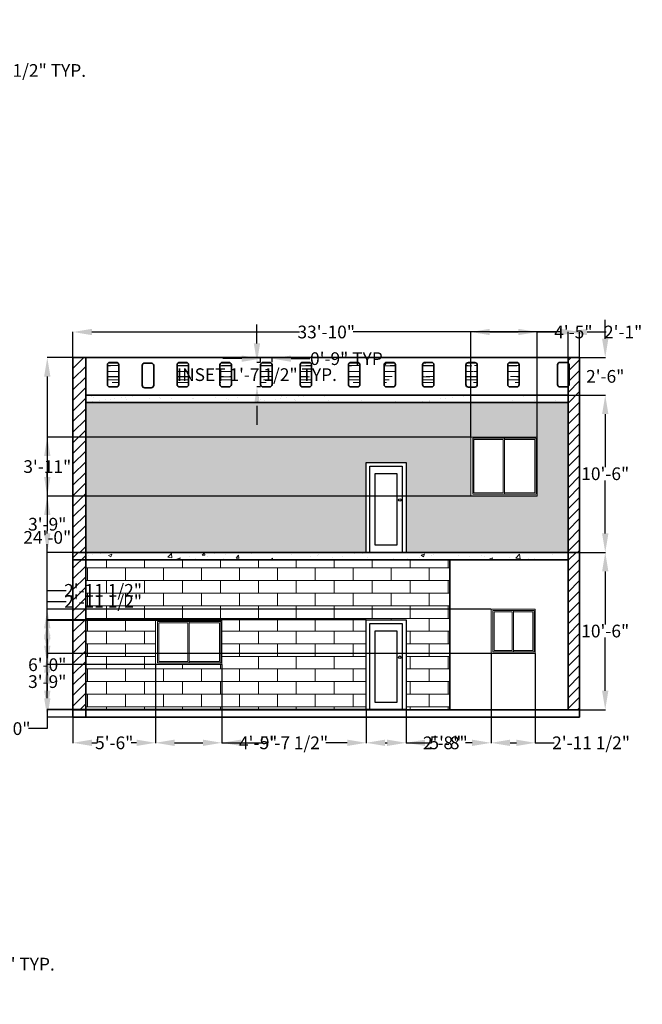
# Model space of a CAD drawing. Units: inches. Extents: x -2 to 7298, y -2 to 4583.
# Tile 6 of 6: x 6799 to 7298, y 3778 to 4567. Entities that reach past the tile are written whole.
import ezdxf

# ---------------------------------------------------------------- set-up
doc = ezdxf.new("R2010")
doc.units = ezdxf.units.IN
doc.header["$MEASUREMENT"] = 0
for name, color, linetype, lineweight in [('A-ANNO-DIMS', 2, 'Continuous', 18), ('A-ELEV', 7, 'Continuous', 35), ('A-ELEV-DOOR', 4, 'Continuous', 25), ('A-ELEV-GLAZ', 4, 'Continuous', 18), ('A-ELEV-PATT', 252, 'Continuous', 13)]:
    doc.layers.add(name, color=color, linetype=linetype, lineweight=lineweight)
doc.styles.get("Standard").update_dxf_attribs({"font": 'arial.ttf'})
doc.dimstyles.get("Standard").update_dxf_attribs({"dimtxt": 10.18, "dimasz": 15.18, "dimexe": 0.18, "dimexo": 0.0625, "dimgap": 0.09, "dimtad": 0, "dimtih": 1, "dimtoh": 1, "dimdec": 0, "dimzin": 0, "dimdsep": 46, "dimlunit": 3, "dimtxsty": 'Standard', "dimcen": 0.09, "dimadec": 0, "dimazin": 0, "dimtfac": 1, "dimtdec": 0, "dimtofl": 0, "dimtmove": 0, "dimatfit": 3, "dimfxl": 1, "dimtolj": 1, "dimtzin": 0, "dimarcsym": 0})

# ---------------------------------------------------------------- blocks, each defined once
blk = doc.blocks.new('*U14')
for p, q in [((38.1, 38.1), (38.1, 876.3)), ((38.1, 876.3), (682.2, 876.3)), ((682.2, 38.1), (682.2, 876.3)), ((682.2, 876.3), (1326.3, 876.3)), ((1326.3, 876.3), (1326.3, 38.1)), ((682.2, 38.1), (38.1, 38.1)), ((1326.3, 38.1), (682.2, 38.1))]:
    blk.add_line(p, q)
blk.add_lwpolyline([(0, 0), (1350, 0), (1350, 900), (0, 900)], close=True)
for points in [[(656.8, 850.9), (656.8, 63.5), (63.5, 63.5), (63.5, 850.9), (656.8, 850.9)], [(682.2, 850.9), (1300.9, 850.9), (1300.9, 63.5), (682.2, 63.5)]]:
    blk.add_lwpolyline(points)
blk = doc.blocks.new('*U17')
blk.add_lwpolyline([(3.12, 0.01), (0.12, 0.01), (0.12, 72.01), (32.12, 72.01), (32.12, 0.01), (29.12, 0.01)])
for points in [[(29.12, 68.99), (29.12, 0.01), (3.12, 0.01), (3.12, 68.99)], [(25.12, 6.01), (25.12, 62.99), (7.12, 62.99), (7.12, 6.01)]]:
    blk.add_lwpolyline(points, close=True)
blk.add_circle((27.12, 42.01), 1)
blk = doc.blocks.new('*U18')
for p, q in [((38.1, 38.1), (38.1, 876.3)), ((38.1, 876.3), (457.2, 876.3)), ((457.2, 38.1), (457.2, 876.3)), ((457.2, 876.3), (876.3, 876.3)), ((876.3, 876.3), (876.3, 38.1)), ((457.2, 38.1), (38.1, 38.1)), ((876.3, 38.1), (457.2, 38.1))]:
    blk.add_line(p, q)
blk.add_lwpolyline([(0, 0), (900, 0), (900, 900), (0, 900)], close=True)
for points in [[(431.8, 850.9), (431.8, 63.5), (63.5, 63.5), (63.5, 850.9), (431.8, 850.9)], [(457.2, 850.9), (850.9, 850.9), (850.9, 63.5), (457.2, 63.5)]]:
    blk.add_lwpolyline(points)
blk = doc.blocks.new('*U19')
for p, q in [((38.1, 38.1), (38.1, 1176.3)), ((38.1, 1176.3), (682.2, 1176.3)), ((682.2, 38.1), (682.2, 1176.3)), ((682.2, 1176.3), (1326.3, 1176.3)), ((1326.3, 1176.3), (1326.3, 38.1)), ((682.2, 38.1), (38.1, 38.1)), ((1326.3, 38.1), (682.2, 38.1))]:
    blk.add_line(p, q)
blk.add_lwpolyline([(0, 0), (1350, 0), (1350, 1200), (0, 1200)], close=True)
for points in [[(656.8, 1150.9), (656.8, 63.5), (63.5, 63.5), (63.5, 1150.9), (656.8, 1150.9)], [(682.2, 1150.9), (1300.9, 1150.9), (1300.9, 63.5), (682.2, 63.5)]]:
    blk.add_lwpolyline(points)
blk = doc.blocks.new('PARAPET-INSET')
blk.add_lwpolyline([(0, 17.72, -0.414214), (2, 19.72), (7.14, 19.72, -0.414214), (9.14, 17.72), (9.14, 2, -0.414214), (7.14, 0), (2, 0, -0.414214), (0, 2)], format="xyb", close=True)
blk = doc.blocks.new('*D33')
at = {"layer": 'A-ANNO-DIMS', "color": 0, "lineweight": -2, "transparency": 16777216}
for p, q in [((6989.04, 4307.74), (6989.04, 4322.92)), ((6991.93, 4292.56), (6988.86, 4292.56)), ((6991.93, 4272.84), (6988.86, 4272.84)), ((6989.04, 4257.66), (6989.04, 4242.48))]:
    blk.add_line(p, q, dxfattribs=at)
at = {"layer": 'A-ANNO-DIMS', "color": 0, "transparency": 16777216}
for points in [[(6986.51, 4307.74), (6991.57, 4307.74), (6989.04, 4292.56)], [(6986.51, 4257.66), (6991.57, 4257.66), (6989.04, 4272.84)]]:
    blk.add_solid(points, dxfattribs=at)
at = {"layer": 'Defpoints', "color": 0, "transparency": 16777216}
for p in [(6989.04, 4292.56), (6991.99, 4292.56), (6991.99, 4272.84)]:
    blk.add_point(p, dxfattribs=at)
at = {"layer": 'A-ANNO-DIMS', "color": 0, "transparency": 16777216, "insert": (6989.04, 4282.7), "char_height": 10.18, "attachment_point": 5}
blk.add_mtext('\\A1;INSET 1\'-7 1/2" TYP.', dxfattribs=at)
blk = doc.blocks.new('*D34')
at = {"layer": 'A-ANNO-DIMS', "color": 0, "lineweight": -2, "transparency": 16777216}
for p, q in [((6976.81, 4295.52), (6961.63, 4295.52)), ((6991.99, 4292.62), (6991.99, 4295.7)), ((7001.14, 4292.62), (7001.14, 4295.7)), ((7016.32, 4295.52), (7031.5, 4295.52))]:
    blk.add_line(p, q, dxfattribs=at)
at = {"layer": 'A-ANNO-DIMS', "color": 0, "transparency": 16777216}
for points in [[(6976.81, 4298.05), (6976.81, 4292.99), (6991.99, 4295.52)], [(7016.32, 4298.05), (7016.32, 4292.99), (7001.14, 4295.52)]]:
    blk.add_solid(points, dxfattribs=at)
at = {"layer": 'Defpoints', "color": 0, "transparency": 16777216}
for p in [(6991.99, 4292.56), (7001.14, 4295.52), (7001.14, 4292.56)]:
    blk.add_point(p, dxfattribs=at)
at = {"layer": 'A-ANNO-DIMS', "color": 0, "transparency": 16777216, "insert": (7062.62, 4295.52), "char_height": 10.18, "attachment_point": 5}
blk.add_mtext('\\A1;0\'-9" TYP.', dxfattribs=at)
blk = doc.blocks.new('*D45')
at = {"layer": 'A-ANNO-DIMS', "color": 0, "lineweight": -2, "transparency": 16777216}
for p, q in [((6628.99, 3810.47), (6613.81, 3810.47)), ((6644.17, 3809.69), (6644.17, 3810.65)), ((6649.81, 3809.69), (6649.81, 3810.65)), ((6664.99, 3810.47), (6680.17, 3810.47))]:
    blk.add_line(p, q, dxfattribs=at)
at = {"layer": 'A-ANNO-DIMS', "color": 0, "transparency": 16777216}
for points in [[(6628.99, 3813), (6628.99, 3807.94), (6644.17, 3810.47)], [(6664.99, 3813), (6664.99, 3807.94), (6649.81, 3810.47)]]:
    blk.add_solid(points, dxfattribs=at)
at = {"layer": 'Defpoints', "color": 0, "transparency": 16777216}
for p in [(6649.81, 3810.47), (6644.17, 3809.63), (6649.81, 3809.63)]:
    blk.add_point(p, dxfattribs=at)
at = {"layer": 'A-ANNO-DIMS', "color": 0, "transparency": 16777216, "insert": (6754.93, 3810.47), "char_height": 10.18, "attachment_point": 5}
blk.add_mtext('\\A1;BURNER 0\'-5 1/2" TYP.', dxfattribs=at)
blk = doc.blocks.new('*D53')
at = {"layer": 'A-ANNO-DIMS', "color": 0, "lineweight": -2, "transparency": 16777216}
for p, q in [((6616.96, 4528.32), (6616.96, 4526.19)), ((6630.33, 4528.32), (6630.33, 4526.19)), ((6601.78, 4526.37), (6586.6, 4526.37)), ((6645.51, 4526.37), (6660.69, 4526.37))]:
    blk.add_line(p, q, dxfattribs=at)
at = {"layer": 'A-ANNO-DIMS', "color": 0, "transparency": 16777216}
for points in [[(6601.78, 4528.9), (6601.78, 4523.84), (6616.96, 4526.37)], [(6645.51, 4528.9), (6645.51, 4523.84), (6630.33, 4526.37)]]:
    blk.add_solid(points, dxfattribs=at)
at = {"layer": 'Defpoints', "color": 0, "transparency": 16777216}
for p in [(6616.96, 4528.38), (6630.33, 4528.38), (6630.33, 4526.37)]:
    blk.add_point(p, dxfattribs=at)
at = {"layer": 'A-ANNO-DIMS', "color": 0, "transparency": 16777216, "insert": (6758.34, 4526.37), "char_height": 10.18, "attachment_point": 5}
blk.add_mtext('\\A1;NIGHTSTAND A 1\'-1 1/2" TYP.', dxfattribs=at)
blk = doc.blocks.new('*D72')
at = {"layer": 'A-ANNO-DIMS', "color": 0, "lineweight": -2, "transparency": 16777216}
for p, q in [((6841.6, 4296.38), (6841.6, 4317.05)), ((6856.78, 4316.87), (7023.03, 4316.87)), ((7232.33, 4316.87), (7066.08, 4316.87)), ((7247.51, 4296.38), (7247.51, 4317.05))]:
    blk.add_line(p, q, dxfattribs=at)
at = {"layer": 'A-ANNO-DIMS', "color": 0, "transparency": 16777216}
for points in [[(6856.78, 4319.4), (6856.78, 4314.34), (6841.6, 4316.87)], [(7232.33, 4319.4), (7232.33, 4314.34), (7247.51, 4316.87)]]:
    blk.add_solid(points, dxfattribs=at)
at = {"layer": 'Defpoints', "color": 0, "transparency": 16777216}
for p in [(7247.51, 4316.87), (6841.6, 4296.32), (7247.51, 4296.32)]:
    blk.add_point(p, dxfattribs=at)
at = {"layer": 'A-ANNO-DIMS', "color": 0, "transparency": 16777216, "insert": (7044.55, 4316.87), "char_height": 10.18, "attachment_point": 5}
blk.add_mtext('\\A1;33\'-10"', dxfattribs=at)
blk = doc.blocks.new('*D73')
at = {"layer": 'A-ANNO-DIMS', "color": 0, "lineweight": -2, "transparency": 16777216}
for p, q in [((6841.54, 4296.32), (6820.87, 4296.32)), ((6821.05, 4281.14), (6821.05, 4157.6)), ((6821.05, 4023.5), (6821.05, 4147.03)), ((6841.54, 4008.32), (6820.87, 4008.32))]:
    blk.add_line(p, q, dxfattribs=at)
at = {"layer": 'A-ANNO-DIMS', "color": 0, "transparency": 16777216}
for points in [[(6818.52, 4281.14), (6823.58, 4281.14), (6821.05, 4296.32)], [(6818.52, 4023.5), (6823.58, 4023.5), (6821.05, 4008.32)]]:
    blk.add_solid(points, dxfattribs=at)
at = {"layer": 'Defpoints', "color": 0, "transparency": 16777216}
for p in [(6821.05, 4296.32), (6841.6, 4296.32), (6841.6, 4008.32)]:
    blk.add_point(p, dxfattribs=at)
at = {"layer": 'A-ANNO-DIMS', "color": 0, "transparency": 16777216, "insert": (6821.05, 4152.32), "char_height": 10.18, "attachment_point": 5}
blk.add_mtext('\\A1;24\'-0"', dxfattribs=at)
blk = doc.blocks.new('*D74')
at = {"layer": 'A-ANNO-DIMS', "color": 0, "lineweight": -2, "transparency": 16777216}
for p, q in [((7247.57, 4140.32), (7268.24, 4140.32)), ((7268.06, 4125.14), (7268.06, 4082.6)), ((7268.06, 4029.5), (7268.06, 4072.03)), ((7247.57, 4014.32), (7268.24, 4014.32))]:
    blk.add_line(p, q, dxfattribs=at)
at = {"layer": 'A-ANNO-DIMS', "color": 0, "transparency": 16777216}
for points in [[(7265.53, 4125.14), (7270.59, 4125.14), (7268.06, 4140.32)], [(7265.53, 4029.5), (7270.59, 4029.5), (7268.06, 4014.32)]]:
    blk.add_solid(points, dxfattribs=at)
at = {"layer": 'Defpoints', "color": 0, "transparency": 16777216}
for p in [(7247.51, 4140.32), (7268.06, 4140.32), (7247.51, 4014.32)]:
    blk.add_point(p, dxfattribs=at)
at = {"layer": 'A-ANNO-DIMS', "color": 0, "transparency": 16777216, "insert": (7268.06, 4077.32), "char_height": 10.18, "attachment_point": 5}
blk.add_mtext('\\A1;10\'-6"', dxfattribs=at)
blk = doc.blocks.new('*D75')
at = {"layer": 'A-ANNO-DIMS', "color": 0, "lineweight": -2, "transparency": 16777216}
for p, q in [((7238.41, 4266.32), (7268.24, 4266.32)), ((7268.06, 4251.14), (7268.06, 4208.6)), ((7268.06, 4155.5), (7268.06, 4198.03)), ((7247.57, 4140.32), (7268.24, 4140.32))]:
    blk.add_line(p, q, dxfattribs=at)
at = {"layer": 'A-ANNO-DIMS', "color": 0, "transparency": 16777216}
for points in [[(7265.53, 4251.14), (7270.59, 4251.14), (7268.06, 4266.32)], [(7265.53, 4155.5), (7270.59, 4155.5), (7268.06, 4140.32)]]:
    blk.add_solid(points, dxfattribs=at)
at = {"layer": 'Defpoints', "color": 0, "transparency": 16777216}
for p in [(7238.34, 4266.32), (7268.06, 4266.32), (7247.51, 4140.32)]:
    blk.add_point(p, dxfattribs=at)
at = {"layer": 'A-ANNO-DIMS', "color": 0, "transparency": 16777216, "insert": (7268.06, 4203.32), "char_height": 10.18, "attachment_point": 5}
blk.add_mtext('\\A1;10\'-6"', dxfattribs=at)
blk = doc.blocks.new('*D76')
at = {"layer": 'A-ANNO-DIMS', "color": 0, "lineweight": -2, "transparency": 16777216}
for p, q in [((7268.05558, 4311.496026), (7268.05558, 4326.676026)), ((7247.56808, 4296.316026), (7268.23558, 4296.316026)), ((7238.406619, 4266.316026), (7268.23558, 4266.316026)), ((7268.05558, 4251.136026), (7268.05558, 4235.956026))]:
    blk.add_line(p, q, dxfattribs=at)
at = {"layer": 'A-ANNO-DIMS', "color": 0, "transparency": 16777216}
for points in [[(7265.52558, 4311.496026), (7270.58558, 4311.496026), (7268.05558, 4296.316026)], [(7265.52558, 4251.136026), (7270.58558, 4251.136026), (7268.05558, 4266.316026)]]:
    blk.add_solid(points, dxfattribs=at)
at = {"layer": 'Defpoints', "color": 0, "transparency": 16777216}
for p in [(7247.50558, 4296.316026), (7268.05558, 4296.316026), (7238.344119, 4266.316026)]:
    blk.add_point(p, dxfattribs=at)
at = {"layer": 'A-ANNO-DIMS', "color": 0, "transparency": 16777216, "insert": (7268.05558, 4281.316026), "char_height": 10.18, "attachment_point": 5}
blk.add_mtext('\\A1;2\'-6"', dxfattribs=at)
blk = doc.blocks.new('*D77')
at = {"layer": 'A-ANNO-DIMS', "color": 0, "lineweight": -2, "transparency": 16777216}
for p, q in [((6907.79, 4050.38), (6907.79, 3987.59)), ((6841.6, 4014.25), (6841.6, 3987.59)), ((6856.78, 3987.77), (6861.08, 3987.77)), ((6892.61, 3987.77), (6888.32, 3987.77))]:
    blk.add_line(p, q, dxfattribs=at)
at = {"layer": 'A-ANNO-DIMS', "color": 0, "transparency": 16777216}
for points in [[(6856.78, 3990.3), (6856.78, 3985.24), (6841.6, 3987.77)], [(6892.61, 3990.3), (6892.61, 3985.24), (6907.79, 3987.77)]]:
    blk.add_solid(points, dxfattribs=at)
at = {"layer": 'Defpoints', "color": 0, "transparency": 16777216}
for p in [(6907.79, 4050.44), (6841.6, 4014.32), (6907.79, 3987.77)]:
    blk.add_point(p, dxfattribs=at)
at = {"layer": 'A-ANNO-DIMS', "color": 0, "transparency": 16777216, "insert": (6874.7, 3987.77), "char_height": 10.18, "attachment_point": 5}
blk.add_mtext('\\A1;5\'-6"', dxfattribs=at)
blk = doc.blocks.new('*D78')
at = {"layer": 'A-ANNO-DIMS', "color": 0, "lineweight": -2, "transparency": 16777216}
for p, q in [((6907.79, 4050.38), (6907.79, 3987.59)), ((6960.94, 4050.38), (6960.94, 3987.59)), ((6922.97, 3987.77), (6945.76, 3987.77)), ((6960.94, 3987.77), (6976.12, 3987.77))]:
    blk.add_line(p, q, dxfattribs=at)
at = {"layer": 'A-ANNO-DIMS', "color": 0, "transparency": 16777216}
for points in [[(6922.97, 3990.3), (6922.97, 3985.24), (6907.79, 3987.77)], [(6945.76, 3990.3), (6945.76, 3985.24), (6960.94, 3987.77)]]:
    blk.add_solid(points, dxfattribs=at)
at = {"layer": 'Defpoints', "color": 0, "transparency": 16777216}
for p in [(6907.79, 4050.44), (6960.94, 4050.44), (6960.94, 3987.77)]:
    blk.add_point(p, dxfattribs=at)
at = {"layer": 'A-ANNO-DIMS', "color": 0, "transparency": 16777216, "insert": (6989.95, 3987.77), "char_height": 10.18, "attachment_point": 5}
blk.add_mtext('\\A1;4\'-5"', dxfattribs=at)
blk = doc.blocks.new('*D79')
at = {"layer": 'A-ANNO-DIMS', "color": 0, "lineweight": -2, "transparency": 16777216}
for p, q in [((6960.94, 4050.38), (6960.94, 3987.59)), ((7076.5, 4014.27), (7076.5, 3987.59)), ((6976.12, 3987.77), (6993.24, 3987.77)), ((7061.32, 3987.77), (7044.2, 3987.77))]:
    blk.add_line(p, q, dxfattribs=at)
at = {"layer": 'A-ANNO-DIMS', "color": 0, "transparency": 16777216}
for points in [[(6976.12, 3990.3), (6976.12, 3985.24), (6960.94, 3987.77)], [(7061.32, 3990.3), (7061.32, 3985.24), (7076.5, 3987.77)]]:
    blk.add_solid(points, dxfattribs=at)
at = {"layer": 'Defpoints', "color": 0, "transparency": 16777216}
for p in [(6960.94, 4050.44), (7076.5, 4014.33), (7076.5, 3987.77)]:
    blk.add_point(p, dxfattribs=at)
at = {"layer": 'A-ANNO-DIMS', "color": 0, "transparency": 16777216, "insert": (7018.72, 3987.77), "char_height": 10.18, "attachment_point": 5}
blk.add_mtext('\\A1;9\'-7 1/2"', dxfattribs=at)
blk = doc.blocks.new('*D80')
at = {"layer": 'A-ANNO-DIMS', "color": 0, "lineweight": -2, "transparency": 16777216}
for p, q in [((7076.5, 4014.27), (7076.5, 3987.59)), ((7108.5, 4014.27), (7108.5, 3987.59)), ((7091.68, 3987.77), (7093.32, 3987.77)), ((7108.5, 3987.77), (7123.68, 3987.77))]:
    blk.add_line(p, q, dxfattribs=at)
at = {"layer": 'A-ANNO-DIMS', "color": 0, "transparency": 16777216}
for points in [[(7091.68, 3990.3), (7091.68, 3985.24), (7076.5, 3987.77)], [(7093.32, 3990.3), (7093.32, 3985.24), (7108.5, 3987.77)]]:
    blk.add_solid(points, dxfattribs=at)
at = {"layer": 'Defpoints', "color": 0, "transparency": 16777216}
for p in [(7076.5, 4014.33), (7108.5, 4014.33), (7108.5, 3987.77)]:
    blk.add_point(p, dxfattribs=at)
at = {"layer": 'A-ANNO-DIMS', "color": 0, "transparency": 16777216, "insert": (7137.39, 3987.77), "char_height": 10.18, "attachment_point": 5}
blk.add_mtext('\\A1;2\'-8"', dxfattribs=at)
blk = doc.blocks.new('*D81')
at = {"layer": 'A-ANNO-DIMS', "color": 0, "lineweight": -2, "transparency": 16777216}
for p, q in [((7176.58, 4059.21), (7176.58, 3987.59)), ((7108.5, 4014.27), (7108.5, 3987.59)), ((7123.68, 3987.77), (7128.92, 3987.77)), ((7161.4, 3987.77), (7156.16, 3987.77))]:
    blk.add_line(p, q, dxfattribs=at)
at = {"layer": 'A-ANNO-DIMS', "color": 0, "transparency": 16777216}
for points in [[(7123.68, 3990.3), (7123.68, 3985.24), (7108.5, 3987.77)], [(7161.4, 3990.3), (7161.4, 3985.24), (7176.58, 3987.77)]]:
    blk.add_solid(points, dxfattribs=at)
at = {"layer": 'Defpoints', "color": 0, "transparency": 16777216}
for p in [(7176.58, 4059.27), (7108.5, 4014.33), (7176.58, 3987.77)]:
    blk.add_point(p, dxfattribs=at)
at = {"layer": 'A-ANNO-DIMS', "color": 0, "transparency": 16777216, "insert": (7142.54, 3987.77), "char_height": 10.18, "attachment_point": 5}
blk.add_mtext('\\A1;5\'-8"', dxfattribs=at)
blk = doc.blocks.new('*D82')
at = {"layer": 'A-ANNO-DIMS', "color": 0, "lineweight": -2, "transparency": 16777216}
for p, q in [((7176.58, 4059.21), (7176.58, 3987.59)), ((7212.02, 4059.21), (7212.02, 3987.59)), ((7191.76, 3987.77), (7196.84, 3987.77)), ((7212.02, 3987.77), (7227.2, 3987.77))]:
    blk.add_line(p, q, dxfattribs=at)
at = {"layer": 'A-ANNO-DIMS', "color": 0, "transparency": 16777216}
for points in [[(7191.76, 3990.3), (7191.76, 3985.24), (7176.58, 3987.77)], [(7196.84, 3990.3), (7196.84, 3985.24), (7212.02, 3987.77)]]:
    blk.add_solid(points, dxfattribs=at)
at = {"layer": 'Defpoints', "color": 0, "transparency": 16777216}
for p in [(7176.58, 4059.27), (7212.02, 4059.27), (7212.02, 3987.77)]:
    blk.add_point(p, dxfattribs=at)
at = {"layer": 'A-ANNO-DIMS', "color": 0, "transparency": 16777216, "insert": (7256.72, 3987.77), "char_height": 10.18, "attachment_point": 5}
blk.add_mtext('\\A1;2\'-11 1/2"', dxfattribs=at)
blk = doc.blocks.new('*D83')
at = {"layer": 'A-ANNO-DIMS', "color": 0, "lineweight": -2, "transparency": 16777216}
for p, q in [((6821.05, 4085.87), (6821.05, 4101.05)), ((6821.05, 4101.05), (6836.23, 4101.05)), ((6907.73, 4085.87), (6820.87, 4085.87)), ((6821.05, 4065.62), (6821.05, 4070.69)), ((6907.73, 4050.44), (6820.87, 4050.44))]:
    blk.add_line(p, q, dxfattribs=at)
at = {"layer": 'A-ANNO-DIMS', "color": 0, "transparency": 16777216}
for points in [[(6818.52, 4070.69), (6823.58, 4070.69), (6821.05, 4085.87)], [(6818.52, 4065.62), (6823.58, 4065.62), (6821.05, 4050.44)]]:
    blk.add_solid(points, dxfattribs=at)
at = {"layer": 'Defpoints', "color": 0, "transparency": 16777216}
for p in [(6821.05, 4085.87), (6907.79, 4085.87), (6907.79, 4050.44)]:
    blk.add_point(p, dxfattribs=at)
at = {"layer": 'A-ANNO-DIMS', "color": 0, "transparency": 16777216, "insert": (6865.76, 4101.05), "char_height": 10.18, "attachment_point": 5}
blk.add_mtext('\\A1;2\'-11 1/2"', dxfattribs=at)
blk = doc.blocks.new('*D84')
at = {"layer": 'A-ANNO-DIMS', "color": 0, "lineweight": -2, "transparency": 16777216}
for p, q in [((6960.88, 4050.44), (6820.87, 4050.44)), ((6821.05, 4035.26), (6821.05, 4029.51)), ((7076.44, 4014.33), (6820.87, 4014.33)), ((6821.05, 4014.33), (6821.05, 3999.15)), ((6821.05, 3999.15), (6805.87, 3999.15))]:
    blk.add_line(p, q, dxfattribs=at)
at = {"layer": 'A-ANNO-DIMS', "color": 0, "transparency": 16777216}
for points in [[(6818.52, 4035.26), (6823.58, 4035.26), (6821.05, 4050.44)], [(6818.52, 4029.51), (6823.58, 4029.51), (6821.05, 4014.33)]]:
    blk.add_solid(points, dxfattribs=at)
at = {"layer": 'Defpoints', "color": 0, "transparency": 16777216}
for p in [(6960.94, 4050.44), (6821.05, 4014.33), (7076.5, 4014.33)]:
    blk.add_point(p, dxfattribs=at)
at = {"layer": 'A-ANNO-DIMS', "color": 0, "transparency": 16777216, "insert": (6792.26, 3999.15), "char_height": 10.18, "attachment_point": 5}
blk.add_mtext('\\A1;3\'-0"', dxfattribs=at)
blk = doc.blocks.new('*D85')
at = {"layer": 'A-ANNO-DIMS', "color": 0, "lineweight": -2, "transparency": 16777216}
for p, q in [((7076.44, 4086.33), (6820.87, 4086.33)), ((6821.05, 4071.15), (6821.05, 4055.62)), ((6821.05, 4029.51), (6821.05, 4045.04)), ((7076.44, 4014.33), (6820.87, 4014.33))]:
    blk.add_line(p, q, dxfattribs=at)
at = {"layer": 'A-ANNO-DIMS', "color": 0, "transparency": 16777216}
for points in [[(6818.52, 4071.15), (6823.58, 4071.15), (6821.05, 4086.33)], [(6818.52, 4029.51), (6823.58, 4029.51), (6821.05, 4014.33)]]:
    blk.add_solid(points, dxfattribs=at)
at = {"layer": 'Defpoints', "color": 0, "transparency": 16777216}
for p in [(6821.05, 4086.33), (7076.5, 4086.33), (7076.5, 4014.33)]:
    blk.add_point(p, dxfattribs=at)
at = {"layer": 'A-ANNO-DIMS', "color": 0, "transparency": 16777216, "insert": (6821.05, 4050.33), "char_height": 10.18, "attachment_point": 5}
blk.add_mtext('\\A1;6\'-0"', dxfattribs=at)
blk = doc.blocks.new('*D86')
at = {"layer": 'A-ANNO-DIMS', "color": 0, "lineweight": -2, "transparency": 16777216}
for p, q in [((6821.05, 4094.71), (6821.05, 4109.89)), ((6821.05, 4109.89), (6836.23, 4109.89)), ((7176.52, 4094.71), (6820.87, 4094.71)), ((6821.05, 4074.45), (6821.05, 4079.53)), ((7176.52, 4059.27), (6820.87, 4059.27))]:
    blk.add_line(p, q, dxfattribs=at)
at = {"layer": 'A-ANNO-DIMS', "color": 0, "transparency": 16777216}
for points in [[(6818.52, 4079.53), (6823.58, 4079.53), (6821.05, 4094.71)], [(6818.52, 4074.45), (6823.58, 4074.45), (6821.05, 4059.27)]]:
    blk.add_solid(points, dxfattribs=at)
at = {"layer": 'Defpoints', "color": 0, "transparency": 16777216}
for p in [(6821.05, 4094.71), (7176.58, 4094.71), (7176.58, 4059.27)]:
    blk.add_point(p, dxfattribs=at)
at = {"layer": 'A-ANNO-DIMS', "color": 0, "transparency": 16777216, "insert": (6865.76, 4109.89), "char_height": 10.18, "attachment_point": 5}
blk.add_mtext('\\A1;2\'-11 1/2"', dxfattribs=at)
blk = doc.blocks.new('*D87')
at = {"layer": 'A-ANNO-DIMS', "color": 0, "lineweight": -2, "transparency": 16777216}
for p, q in [((7211.95, 4059.27), (6820.87, 4059.27)), ((6821.05, 4044.09), (6821.05, 4042.09)), ((6821.05, 4029.5), (6821.05, 4031.5)), ((7238.28, 4014.32), (6820.87, 4014.32))]:
    blk.add_line(p, q, dxfattribs=at)
at = {"layer": 'A-ANNO-DIMS', "color": 0, "transparency": 16777216}
for points in [[(6818.52, 4044.09), (6823.58, 4044.09), (6821.05, 4059.27)], [(6818.52, 4029.5), (6823.58, 4029.5), (6821.05, 4014.32)]]:
    blk.add_solid(points, dxfattribs=at)
at = {"layer": 'Defpoints', "color": 0, "transparency": 16777216}
for p in [(7212.02, 4059.27), (6821.05, 4014.32), (7238.34, 4014.32)]:
    blk.add_point(p, dxfattribs=at)
at = {"layer": 'A-ANNO-DIMS', "color": 0, "transparency": 16777216, "insert": (6821.05, 4036.8), "char_height": 10.18, "attachment_point": 5}
blk.add_mtext('\\A1;3\'-9"', dxfattribs=at)
blk = doc.blocks.new('*D88')
at = {"layer": 'A-ANNO-DIMS', "color": 0, "lineweight": -2, "transparency": 16777216}
for p, q in [((7160.31, 4232.68), (6820.87, 4232.68)), ((6821.05, 4217.5), (6821.05, 4214.35)), ((6821.05, 4200.62), (6821.05, 4203.77)), ((7160.31, 4185.44), (6820.87, 4185.44))]:
    blk.add_line(p, q, dxfattribs=at)
at = {"layer": 'A-ANNO-DIMS', "color": 0, "transparency": 16777216}
for points in [[(6818.52, 4217.5), (6823.58, 4217.5), (6821.05, 4232.68)], [(6818.52, 4200.62), (6823.58, 4200.62), (6821.05, 4185.44)]]:
    blk.add_solid(points, dxfattribs=at)
at = {"layer": 'Defpoints', "color": 0, "transparency": 16777216}
for p in [(6821.05, 4232.68), (7160.38, 4232.68), (7160.38, 4185.44)]:
    blk.add_point(p, dxfattribs=at)
at = {"layer": 'A-ANNO-DIMS', "color": 0, "transparency": 16777216, "insert": (6821.05, 4209.06), "char_height": 10.18, "attachment_point": 5}
blk.add_mtext('\\A1;3\'-11"', dxfattribs=at)
blk = doc.blocks.new('*D89')
at = {"layer": 'A-ANNO-DIMS', "color": 0, "lineweight": -2, "transparency": 16777216}
for p, q in [((7213.46, 4185.44), (6820.87, 4185.44)), ((6821.05, 4170.26), (6821.05, 4168.17)), ((6821.05, 4155.5), (6821.05, 4157.59)), ((7238.28, 4140.32), (6820.87, 4140.32))]:
    blk.add_line(p, q, dxfattribs=at)
at = {"layer": 'A-ANNO-DIMS', "color": 0, "transparency": 16777216}
for points in [[(6818.52, 4170.26), (6823.58, 4170.26), (6821.05, 4185.44)], [(6818.52, 4155.5), (6823.58, 4155.5), (6821.05, 4140.32)]]:
    blk.add_solid(points, dxfattribs=at)
at = {"layer": 'Defpoints', "color": 0, "transparency": 16777216}
for p in [(7213.53, 4185.44), (6821.05, 4140.32), (7238.34, 4140.32)]:
    blk.add_point(p, dxfattribs=at)
at = {"layer": 'A-ANNO-DIMS', "color": 0, "transparency": 16777216, "insert": (6821.05, 4162.88), "char_height": 10.18, "attachment_point": 5}
blk.add_mtext('\\A1;3\'-9"', dxfattribs=at)
blk = doc.blocks.new('*D90')
at = {"layer": 'A-ANNO-DIMS', "color": 0, "lineweight": -2, "transparency": 16777216}
for p, q in [((7198.35, 4316.87), (7183.17, 4316.87)), ((7213.53, 4232.75), (7213.53, 4317.05)), ((7238.34, 4260.38), (7238.34, 4317.05)), ((7253.52, 4316.87), (7268.7, 4316.87))]:
    blk.add_line(p, q, dxfattribs=at)
at = {"layer": 'A-ANNO-DIMS', "color": 0, "transparency": 16777216}
for points in [[(7198.35, 4319.4), (7198.35, 4314.34), (7213.53, 4316.87)], [(7253.52, 4319.4), (7253.52, 4314.34), (7238.34, 4316.87)]]:
    blk.add_solid(points, dxfattribs=at)
at = {"layer": 'Defpoints', "color": 0, "transparency": 16777216}
for p in [(7238.34, 4316.87), (7238.34, 4260.32), (7213.53, 4232.68)]:
    blk.add_point(p, dxfattribs=at)
at = {"layer": 'A-ANNO-DIMS', "color": 0, "transparency": 16777216, "insert": (7282.41, 4316.87), "char_height": 10.18, "attachment_point": 5}
blk.add_mtext('\\A1;2\'-1"', dxfattribs=at)
blk = doc.blocks.new('*D91')
at = {"layer": 'A-ANNO-DIMS', "color": 0, "lineweight": -2, "transparency": 16777216}
for p, q in [((7160.38, 4232.75), (7160.38, 4317.05)), ((7175.56, 4316.87), (7198.35, 4316.87)), ((7213.53, 4232.75), (7213.53, 4317.05)), ((7213.53, 4316.87), (7228.71, 4316.87))]:
    blk.add_line(p, q, dxfattribs=at)
at = {"layer": 'A-ANNO-DIMS', "color": 0, "transparency": 16777216}
for points in [[(7175.56, 4319.4), (7175.56, 4314.34), (7160.38, 4316.87)], [(7198.35, 4319.4), (7198.35, 4314.34), (7213.53, 4316.87)]]:
    blk.add_solid(points, dxfattribs=at)
at = {"layer": 'Defpoints', "color": 0, "transparency": 16777216}
for p in [(7213.53, 4316.87), (7160.38, 4232.68), (7213.53, 4232.68)]:
    blk.add_point(p, dxfattribs=at)
at = {"layer": 'A-ANNO-DIMS', "color": 0, "transparency": 16777216, "insert": (7242.53, 4316.87), "char_height": 10.18, "attachment_point": 5}
blk.add_mtext('\\A1;4\'-5"', dxfattribs=at)

msp = doc.modelspace()

# ---------------------------------------------------------------- hatches: boundary and pattern name
at = {"layer": 'A-ELEV-PATT'}
h = msp.add_hatch(dxfattribs=at)
h.set_pattern_fill('ANSI31', color=256, scale=48)
h.set_pattern_definition([(45, (-5580.251, -2992.259), (-4.2426407, 4.2426407), [])])
h.paths.add_polyline_path([(6841.6, 4140.32), (6851.82, 4140.32), (6851.82, 4296.32), (6841.6, 4296.32)])
h.paths.add_polyline_path([(7247.51, 4296.32), (7238.34, 4296.32), (7238.34, 4140.32), (7247.51, 4140.32)])
h = msp.add_hatch(dxfattribs=at)
h.set_pattern_fill('AR-RROOF', color=256, scale=6.7)
h.set_pattern_definition([(0, (-5580.251, -3118.259), (14.74, 6.7), [100.5, -13.4, 33.5, -6.7]), (0, (-5571.34, -3114.909), (-6.7, 8.911), [20.1, -2.211, 40.2, -5.025]), (0, (-5576.901, -3112.564), (34.84, 4.489), [53.6, -9.38, 26.8, -6.7])])
h.paths.add_polyline_path([(6925.08, 4290.56, -0.414214), (6927.08, 4292.56), (6932.22, 4292.56, -0.414214), (6934.22, 4290.56), (6934.22, 4274.84, -0.414214), (6932.22, 4272.84), (6927.08, 4272.84, -0.414214), (6925.08, 4274.84)], flags=16)
h.paths.add_polyline_path([(6878.35, 4274.84, -0.414214), (6876.35, 4272.84), (6871.21, 4272.84, -0.414214), (6869.21, 4274.84), (6869.21, 4290.56, -0.414214), (6871.21, 4292.56), (6876.35, 4292.56, -0.414214), (6878.35, 4290.56)], flags=16)
h.paths.add_polyline_path([(6959.38, 4290.56, -0.414214), (6961.38, 4292.56), (6966.52, 4292.56, -0.414214), (6968.52, 4290.56), (6968.52, 4274.84, -0.414214), (6966.52, 4272.84), (6961.38, 4272.84, -0.414214), (6959.38, 4274.84)], flags=16)
h.paths.add_polyline_path([(6991.99, 4290.56, -0.414214), (6993.99, 4292.56), (6999.14, 4292.56, -0.414214), (7001.14, 4290.56), (7001.14, 4274.84, -0.414214), (6999.14, 4272.84), (6993.99, 4272.84, -0.414214), (6991.99, 4274.84)], flags=16)
h.paths.add_polyline_path([(7023.71, 4290.56, -0.414214), (7025.71, 4292.56), (7030.85, 4292.56, -0.414214), (7032.85, 4290.56), (7032.85, 4274.84, -0.414214), (7030.85, 4272.84), (7025.71, 4272.84, -0.414214), (7023.71, 4274.84)], flags=16)
h.paths.add_polyline_path([(7062.33, 4290.56, -0.414214), (7064.33, 4292.56), (7069.48, 4292.56, -0.414214), (7071.48, 4290.56), (7071.48, 4274.84, -0.414214), (7069.48, 4272.84), (7064.33, 4272.84, -0.414214), (7062.33, 4274.84)], flags=16)
h.paths.add_polyline_path([(7090.86, 4290.56, -0.414214), (7092.86, 4292.56), (7098, 4292.56, -0.414214), (7100, 4290.56), (7100, 4274.84, -0.414214), (7098, 4272.84), (7092.86, 4272.84, -0.414214), (7090.86, 4274.84)], flags=16)
h.paths.add_polyline_path([(7121.69, 4290.56, -0.414214), (7123.69, 4292.56), (7128.84, 4292.56, -0.414214), (7130.84, 4290.56), (7130.84, 4274.84, -0.414214), (7128.84, 4272.84), (7123.69, 4272.84, -0.414214), (7121.69, 4274.84)], flags=16)
h.paths.add_polyline_path([(7156.42, 4290.45, -0.414214), (7158.42, 4292.45), (7163.57, 4292.45, -0.414214), (7165.57, 4290.45), (7165.57, 4274.73, -0.414214), (7163.57, 4272.73), (7158.42, 4272.73, -0.414214), (7156.42, 4274.73)], flags=16)
h.paths.add_polyline_path([(7189.95, 4290.56, -0.414214), (7191.95, 4292.56), (7197.1, 4292.56, -0.414214), (7199.1, 4290.56), (7199.1, 4274.84, -0.414214), (7197.1, 4272.84), (7191.95, 4272.84, -0.414214), (7189.95, 4274.84)], flags=16)
h = msp.add_hatch(dxfattribs=at)
h.set_pattern_fill('AR-SAND', color=256, scale=6.7)
h.set_pattern_definition([(37.5, (-5580.251, -3118.259), (-0.4220555, 12.909719), [0, -10.184, 0, -11.39, 0, -10.8875]), (7.5, (-5580.251, -3118.26), (11.857504, 18.908379), [0, -5.494, 0, -9.179, 0, -3.5175]), (327.5, (-5588.492, -3118.259), (20.8647505, 0.037916), [0, -3.35, 0, -12.06, 0, -15.745]), (317.5, (-5588.492, -3118.26), (20.141048, 5.880426), [0, -1.675, 0, -7.906, 0, -9.045])])
h.paths.add_polyline_path([(7238.34, 4266.32), (6851.82, 4266.32), (6851.82, 4260.32), (7238.34, 4260.32)])
h = msp.add_hatch(dxfattribs=at)
h.set_pattern_fill('HONEY', color=256, scale=6.7)
h.set_pattern_definition([(0, (-5580.2512, -3118.2592), (1.25625, 0.725296276), [0.8375, -1.675]), (120, (-5580.2512, -3118.2592), (-1.25625, 0.725296276), [0.8375, -1.675]), (60, (-5580.2512, -3118.2592), (3e-16, 1.45059255), [-1.675, 0.8375])])
h.paths.add_polyline_path([(6851.82, 4260.32), (6851.82, 4140.32), (7076.5, 4140.32), (7076.5, 4212.33), (7108.5, 4212.33), (7108.5, 4140.32), (7238.34, 4140.32), (7238.34, 4260.32)])
h.paths.add_polyline_path([(7160.38, 4232.68), (7213.53, 4232.68), (7213.53, 4185.44), (7160.38, 4185.44)], flags=16)
h.paths.add_polyline_path([(7161.88, 4231.75), (7187.23, 4231.75), (7212.59, 4231.75), (7212.59, 4186.94), (7187.23, 4186.94), (7161.88, 4186.94)], flags=0)
h.paths.add_polyline_path([(7162.88, 4230.75), (7186.23, 4230.75), (7186.23, 4230.75), (7187.23, 4231.75), (7187.23, 4230.75), (7211.59, 4230.75), (7211.59, 4187.94), (7187.23, 4187.94), (7162.88, 4187.94)], flags=0)
h = msp.add_hatch(dxfattribs=at)
h.set_pattern_fill('ANSI31', color=256, scale=48)
h.set_pattern_definition([(45, (-5580.251, -3118.259), (-4.2426407, 4.2426407), [])])
h.paths.add_polyline_path([(6851.82, 4140.32), (6841.6, 4140.32), (6841.6, 4014.32), (6851.82, 4014.32)])
h.paths.add_polyline_path([(7247.51, 4140.32), (7238.34, 4140.32), (7238.34, 4014.32), (7247.51, 4014.32)])
h = msp.add_hatch(dxfattribs=at)
h.set_pattern_fill('AR-CONC', color=256, scale=3.8)
h.set_pattern_definition([(50, (-5580.251, -3118.26), (27.255887, -2.38458), [2.85, -31.35]), (355, (-5580.25, -3118.26), (-5.27255, 28.5833), [2.28, -25.08]), (100.45144, (-5577.98, -3118.458), (21.983336, 26.19872), [2.422127, -26.6434]), (46.1842, (-5580.25, -3110.66), (40.55517, -6.28973), [4.275, -47.025]), (96.63564, (-5576.87, -3111.183), (35.51715, 37.01651), [3.63319, -39.96512]), (351.18416, (-5580.25, -3110.66), (35.51715, 37.01651), [3.42, -37.62]), (21, (-5576.451, -3112.56), (22.682468, -15.299518), [2.85, -31.35]), (326, (-5576.45, -3112.56), (9.24598, 27.5557), [2.28, -25.08]), (71.45144, (-5574.56, -3113.834), (31.92845, 12.256184), [2.422127, -26.6434]), (37.5, (-5580.251, -3118.259), (0.4620745, 12.6499664), [0, -24.776, 0, -25.46, 0, -25.175]), (7.5, (-5580.251, -3118.259), (9.996642, 14.987645), [0, -14.516, 0, -24.206, 0, -9.595]), (327.5, (-5588.725, -3118.259), (20.2852526, -0.857085), [0, -9.5, 0, -29.64, 0, -39.33]), (317.5, (-5592.525, -3118.26), (22.161074, 3.80399), [0, -12.35, 0, -19.684, 0, -27.93])])
h.paths.add_polyline_path([(7238.34, 4140.32), (6851.82, 4140.32), (6851.82, 4134.32), (7238.34, 4134.32)])
h = msp.add_hatch(dxfattribs=at)
h.set_pattern_fill('AR-BRSTD', color=256, scale=3.8)
h.set_pattern_definition([(0, (-5580.251, -3118.259), (0, 10.1346), []), (90, (-5580.251, -3118.259), (-15.2, 10.1346), [10.1346, -10.1346])])
h.paths.add_polyline_path([(6851.82, 4134.32), (6851.82, 4014.32), (7076.5, 4014.32), (7076.5, 4086.33), (7108.5, 4086.33), (7108.5, 4014.32), (7143.52, 4014.32), (7143.52, 4134.32)])
h.paths.add_polyline_path([(6960.94, 4085.87), (6960.94, 4050.44), (6907.79, 4050.44), (6907.79, 4085.87)], flags=16)
h.paths.add_polyline_path([(6934.65, 4084.94), (6960.01, 4084.94), (6960.01, 4051.94), (6934.65, 4051.94), (6909.29, 4051.94), (6909.29, 4084.94)], flags=0)
h.paths.add_polyline_path([(6934.65, 4084.94), (6934.65, 4083.94), (6959.01, 4083.94), (6959.01, 4052.94), (6934.65, 4052.94), (6910.29, 4052.94), (6910.29, 4083.94), (6933.65, 4083.94), (6933.65, 4083.94)], flags=0)

# ---------------------------------------------------------------- linework, layer by layer
at = {"layer": 'A-ELEV'}
for p, q in [((6841.6, 4296.32), (6841.6, 4140.32)), ((6841.6, 4296.32), (7247.51, 4296.32)), ((6851.82, 4296.32), (6851.82, 4140.32)), ((7238.34, 4296.32), (7238.34, 4140.32)), ((7247.51, 4296.32), (7247.51, 4140.32)), ((6851.82, 4266.32), (7238.34, 4266.32)), ((6851.82, 4260.32), (7238.34, 4260.32)), ((6841.6, 4140.32), (6841.6, 4008.32)), ((6841.6, 4140.32), (7247.51, 4140.32)), ((6841.6, 4140.32), (7247.51, 4140.32)), ((6841.6, 4134.32), (7238.34, 4134.32)), ((6851.82, 4140.32), (6851.82, 4008.32)), ((7143.52, 4134.32), (7143.52, 4014.32)), ((7238.34, 4140.32), (7238.34, 4014.32)), ((7247.51, 4140.32), (7247.51, 4008.32)), ((6841.6, 4014.32), (7247.51, 4014.32)), ((6841.6, 4008.32), (7247.51, 4008.32))]:
    msp.add_line(p, q, dxfattribs=at)
for points in [[(6897.14, 4289.94, -0.414214), (6899.14, 4291.94), (6904.29, 4291.94, -0.414214), (6906.29, 4289.94), (6906.29, 4274.22, -0.414214), (6904.29, 4272.22), (6899.14, 4272.22, -0.414214), (6897.14, 4274.22)], [(7090.86, 4290.56, -0.414214), (7092.86, 4292.56), (7098, 4292.56, -0.414214), (7100, 4290.56), (7100, 4274.84, -0.414214), (7098, 4272.84), (7092.86, 4272.84, -0.414214), (7090.86, 4274.84)], [(7121.69, 4290.56, -0.414214), (7123.69, 4292.56), (7128.84, 4292.56, -0.414214), (7130.84, 4290.56), (7130.84, 4274.84, -0.414214), (7128.84, 4272.84), (7123.69, 4272.84, -0.414214), (7121.69, 4274.84)]]:
    msp.add_lwpolyline(points, format="xyb", close=True, dxfattribs=at)

# ---------------------------------------------------------------- block references
for p in [(6869.21, 4272.84), (6925.08, 4272.84), (6959.38, 4272.84), (6991.99, 4272.84), (7023.71, 4272.84), (7062.34, 4272.84), (7156.42, 4272.73), (7189.95, 4272.84), (7229.88, 4272.84)]:
    msp.add_blockref('PARAPET-INSET', p, dxfattribs=at)
at = {"layer": 'A-ELEV-DOOR'}
for p in [(7076.37, 4140.32), (7076.37, 4014.32)]:
    msp.add_blockref('*U17', p, dxfattribs=at)
at = {"layer": 'A-ELEV-GLAZ', "xscale": 0.0393700787401575, "yscale": 0.0393700787401575, "zscale": 0.0393700787401575}
for name, p in [('*U19', (7160.38, 4185.44)), ('*U18', (7176.58, 4059.27)), ('*U14', (6907.79, 4050.44))]:
    msp.add_blockref(name, p, dxfattribs=at)

# ---------------------------------------------------------------- dimensions: what is measured, and where the dimension line sits
at = {"layer": 'A-ANNO-DIMS'}
for base, p1, p2, text, picture, middle in [((6630.33, 4526.37), (6616.96, 4528.38), (6630.33, 4528.38), 'NIGHTSTAND A <> TYP.', '*D53', (6758.34, 4526.37)), ((7001.1391, 4295.518), (6991.9939, 4292.5599), (7001.1391, 4292.5599), '<> TYP.', '*D34', (7062.6152, 4295.518)), ((6649.81, 3810.47), (6644.17, 3809.63), (6649.81, 3809.63), 'BURNER <> TYP.', '*D45', (6754.93, 3810.47))]:
    dim = msp.add_linear_dim(base=base, p1=p1, p2=p2, text=text, dimstyle='Standard', override={"dimdec": 1, "dimlfac": 1, "dimrnd": 0, "dimzin": 1, "dimdsep": 46, "dimlunit": 4, "dimfrac": 2}, dxfattribs=at)
    dim.commit()
    dim.dimension.update_dxf_attribs({"geometry": picture, "text_midpoint": middle})
for base, p1, p2, picture, middle in [((7247.51, 4316.87), (6841.6, 4296.32), (7247.51, 4296.32), '*D72', (7044.55, 4316.87)), ((7213.5255, 4316.866), (7160.3759, 4232.6847), (7213.5255, 4232.6847), '*D91', (7242.5308, 4316.866)), ((7238.34, 4316.87), (7213.53, 4232.68), (7238.34, 4260.32), '*D90', (7282.41, 4316.87)), ((7176.58, 3987.77), (7108.5, 4014.33), (7176.58, 4059.27), '*D81', (7142.54, 3987.77)), ((7212.02, 3987.77), (7176.58, 4059.27), (7212.02, 4059.27), '*D82', (7256.72, 3987.77)), ((6907.79, 3987.77), (6841.6, 4014.32), (6907.79, 4050.44), '*D77', (6874.7, 3987.77)), ((6960.9424, 3987.766), (6907.7928, 4050.4392), (6960.9424, 4050.4392), '*D78', (6989.9478, 3987.766)), ((7076.5, 3987.77), (6960.94, 4050.44), (7076.5, 4014.33), '*D79', (7018.72, 3987.77)), ((7108.5, 3987.77), (7076.5, 4014.33), (7108.5, 4014.33), '*D80', (7137.39, 3987.77))]:
    dim = msp.add_linear_dim(base=base, p1=p1, p2=p2, dimstyle='Standard', override={"dimdec": 1, "dimlfac": 1, "dimrnd": 0, "dimzin": 1, "dimdsep": 46, "dimlunit": 4, "dimfrac": 2}, dxfattribs=at)
    dim.commit()
    dim.dimension.update_dxf_attribs({"geometry": picture, "text_midpoint": middle})
dim = msp.add_linear_dim(base=(6989.04, 4292.56), p1=(6991.99, 4272.84), p2=(6991.99, 4292.56), angle=90, text='INSET <> TYP.', dimstyle='Standard', override={"dimdec": 1, "dimlfac": 1, "dimrnd": 0, "dimzin": 1, "dimdsep": 46, "dimlunit": 4, "dimfrac": 2}, dxfattribs=at)
dim.commit()
dim.dimension.update_dxf_attribs({"geometry": '*D33', "text_midpoint": (6989.04, 4282.7)})
for base, p1, p2, picture, middle in [((7268.06, 4296.32), (7238.34, 4266.32), (7247.51, 4296.32), '*D76', (7268.06, 4281.32)), ((6821.05, 4296.32), (6841.6, 4008.32), (6841.6, 4296.32), '*D73', (6821.05, 4152.32)), ((7268.06, 4266.32), (7247.51, 4140.32), (7238.34, 4266.32), '*D75', (7268.06, 4203.32)), ((6821.05, 4232.68), (7160.38, 4185.44), (7160.38, 4232.68), '*D88', (6821.05, 4209.06)), ((6821.05, 4140.32), (7213.53, 4185.44), (7238.34, 4140.32), '*D89', (6821.05, 4162.88)), ((7268.06, 4140.32), (7247.51, 4014.32), (7247.51, 4140.32), '*D74', (7268.06, 4077.32)), ((6821.05, 4094.71), (7176.58, 4059.27), (7176.58, 4094.71), '*D86', (6865.76, 4109.89)), ((6821.05, 4085.87), (6907.79, 4050.44), (6907.79, 4085.87), '*D83', (6865.76, 4101.05)), ((6821.05, 4086.33), (7076.5, 4014.33), (7076.5, 4086.33), '*D85', (6821.05, 4050.33)), ((6821.0542, 4014.316), (7212.0173, 4059.2743), (7238.3441, 4014.316), '*D87', (6821.0542, 4036.7952)), ((6821.05, 4014.33), (6960.94, 4050.44), (7076.5, 4014.33), '*D84', (6792.26, 3999.15))]:
    dim = msp.add_linear_dim(base=base, p1=p1, p2=p2, angle=90, dimstyle='Standard', override={"dimdec": 1, "dimlfac": 1, "dimrnd": 0, "dimzin": 1, "dimdsep": 46, "dimlunit": 4, "dimfrac": 2}, dxfattribs=at)
    dim.commit()
    dim.dimension.update_dxf_attribs({"geometry": picture, "text_midpoint": middle})

doc.saveas('drawing.dxf')
